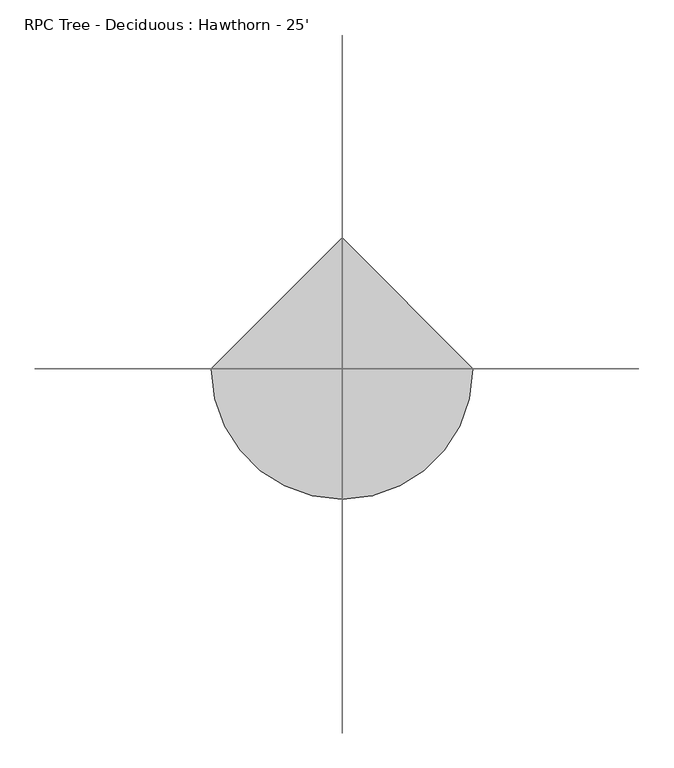
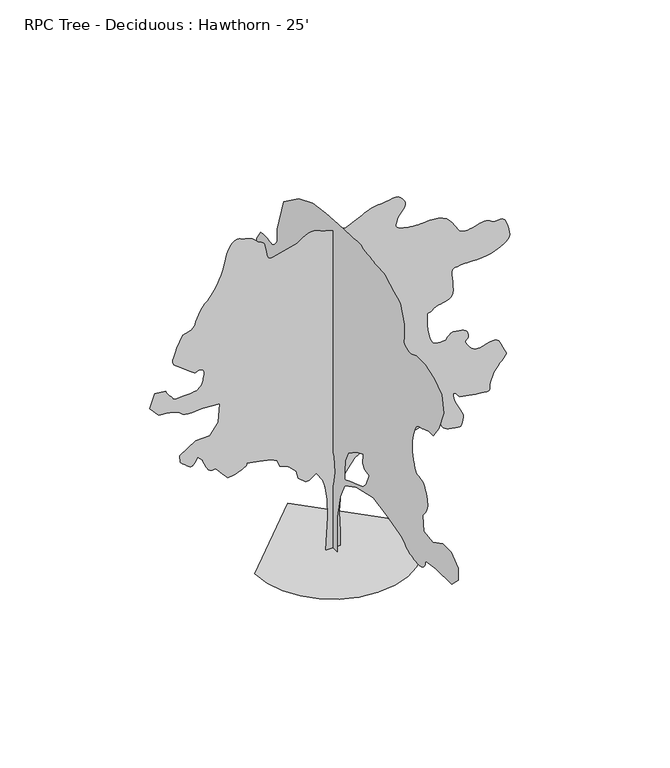
"""IFC4 building model written with IfcOpenShell, lengths in millimetres: geographic element geometry, RPC Tree - Deciduous : Hawthorn - 25'."""

from ifc_helpers import new_model, si_unit, origin, place, context, project, spatial, triangles, source, transform, mapped, element, save


def rpc_tree_deciduous_hawthorn_25_a438f522(model_context):
    return source(origin(), model_context, "Body", "Tessellation", [
        triangles([(159.1331283, 0.0003947, 0.019308), (-154.090976, 0.0003947, 0.019308), (-109.3440979, 0.0003507, 738.3315319), (-120.5310059, 0.000328, 1118.6758307), (-165.2768666, 0.0003107, 1409.5258827), (-210.0237538, 0.0003, 1588.5119053), (-355.4472356, 0.000288, 1789.8701088), (-500.8748051, 0.000294, 1689.1897717), (-579.1803815, 0.0002947, 1678.0035358), (-735.7915707, 0.0002867, 1812.2424351), (-780.538694, 0.000276, 1991.2284576), (-937.1498468, 0.0002667, 2147.8396832), (-1127.3219599, 0.000262, 2226.1452232), (-1183.2552464, 0.000254, 2360.3841225), (-1306.3080551, 0.00025, 2427.5035721), (-1563.5970016, 0.0002467, 2483.4367859), (-1820.8885643, 0.000244, 2528.1814384), (-1818.86674, 0.0002446, 2518.4962738), (-1819.0953598, 0.0002452, 2508.2221916), (-1823.8248676, 0.0002459, 2496.7743439), (-1835.3057076, 0.0002466, 2483.5664291), (-1855.7857075, 0.0002476, 2468.0089485), (-1887.5203983, 0.0002487, 2449.5176353), (-1932.7551373, 0.00025, 2427.5035721), (-1983.2071449, 0.0002513, 2406.1420853), (-2029.5519905, 0.0002523, 2389.4746433), (-2072.4703011, 0.000253, 2376.7238228), (-2112.6530228, 0.0002536, 2367.102317), (-2150.7784573, 0.000254, 2359.8303772), (-2187.5321732, 0.0002544, 2354.1230221), (-2223.605262, 0.0002547, 2349.1978867), (-2346.6579254, 0.0002467, 2483.4367859), (-2480.8968246, 0.0002373, 2640.0478661), (-2507.2492859, 0.0002376, 2635.5522102), (-2533.5026253, 0.0002377, 2632.8090637), (-2559.5553955, 0.0002377, 2633.596225), (-2585.33638, 0.0002373, 2639.6670753), (-2610.710994, 0.0002366, 2652.7732521), (-2635.5774994, 0.0002353, 2674.6934258), (-2659.885318, 0.0002333, 2707.1548164), (-2681.9072296, 0.0002311, 2744.2133102), (-2700.3982521, 0.000229, 2778.9097389), (-2715.9429428, 0.0002271, 2811.6501823), (-2729.1511482, 0.0002252, 2842.8413017), (-2740.6065536, 0.0002234, 2872.8385986), (-2750.8681366, 0.0002217, 2902.0740234), (-2760.570742, 0.00022, 2930.9030777), (-2861.2308769, 0.000214, 3031.5885017), (-2928.3631165, 0.00022, 2930.9030777), (-2940.4789467, 0.0002211, 2912.005394), (-2953.5089653, 0.0002221, 2894.8857994), (-2968.2664948, 0.0002229, 2881.2968033), (-2985.6907219, 0.0002234, 2872.9656258), (-3006.6202583, 0.0002235, 2871.6956451), (-3031.9695831, 0.0002231, 2879.2396614), (-3062.6020157, 0.000222, 2897.3496025), (-3096.5362816, 0.0002205, 2923.0035599), (-3130.1150459, 0.0002188, 2950.6387917), (-3161.5093506, 0.0002172, 2978.0708382), (-3189.0175552, 0.0002157, 3003.1405289), (-3210.8362816, 0.0002144, 3023.7145638), (-3225.212439, 0.0002136, 3037.6337723), (-3230.3940994, 0.0002133, 3042.7645638), (-3241.5701614, 0.000204, 3199.3808762), (-2905.9857033, 0.0001913, 3411.9277863), (-2603.9547203, 0.0001906, 3423.1038483), (-2424.9634655, 0.0001766, 3658.0281715), (-2391.402578, 0.0001526, 4060.7448692), (-2760.570742, 0.0001506, 4094.2980537), (-2839.3868614, 0.0001512, 4085.027108), (-2916.5522095, 0.0001516, 4077.7374367), (-2990.3898537, 0.0001518, 4074.3338654), (-3059.2490227, 0.0001517, 4076.8229576), (-3121.4283669, 0.0001511, 4087.1354095), (-3175.301532, 0.0001499, 4107.2266251), (-3219.2180374, 0.000148, 4139.0528801), (-3263.4394661, 0.0001459, 4173.1650421), (-3318.227401, 0.0001444, 4199.6317406), (-3381.8287514, 0.0001432, 4219.7741158), (-3452.4660095, 0.0001423, 4234.8106979), (-3528.3866661, 0.0001416, 4246.0120491), (-3607.8379211, 0.0001411, 4254.6990189), (-3689.0413948, 0.0001406, 4262.0904282), (-3879.2111824, 0.000128, 4474.6373383), (-3767.3496964, 0.0001106, 4765.4925499), (-3543.6267242, 0.000112, 4743.1151367), (-3529.174118, 0.0001135, 4716.8007545), (-3514.3404305, 0.0001151, 4690.7657158), (-3498.7195816, 0.0001166, 4665.3402328), (-3481.9046196, 0.0001181, 4640.7786507), (-3463.5406242, 0.0001195, 4617.3853111), (-3443.2206436, 0.0001208, 4595.4904266), (-3420.563887, 0.000122, 4575.3227623), (-3403.5713196, 0.0001231, 4556.2983421), (-3395.5956436, 0.0001242, 4538.2642685), (-3389.1692917, 0.0001251, 4522.1861801), (-3376.875856, 0.0001259, 4509.0544235), (-3351.2727676, 0.0001265, 4499.8340561), (-3304.9177483, 0.0001267, 4495.4907166), (-3230.3940994, 0.0001266, 4497.0147514), (-3147.7933273, 0.0001263, 4501.8153305), (-3080.4326134, 0.0001261, 4506.6159096), (-3025.7972855, 0.0001258, 4511.3911995), (-2981.3473824, 0.0001255, 4516.1917786), (-2944.5429428, 0.0001252, 4520.9923576), (-2912.7928459, 0.0001249, 4525.7929367), (-2883.6082901, 0.0001246, 4530.5679359), (-2855.0332901, 0.0001233, 4552.2596352), (-2827.6521126, 0.000122, 4574.6370483), (-2802.607711, 0.0001206, 4598.3858894), (-2781.0686188, 0.0001191, 4624.1668739), (-2764.2539474, 0.0001174, 4652.7165848), (-2753.2810707, 0.0001154, 4684.6695763), (-2749.3693909, 0.0001133, 4720.7377235), (-2745.4071327, 0.0001109, 4760.7934181), (-2736.720163, 0.0001084, 4802.805098), (-2728.2366692, 0.0001059, 4844.6133018), (-2724.858387, 0.0001036, 4884.0850204), (-2731.4370552, 0.0001015, 4919.0352127), (-2752.8999893, 9.98e-05, 4947.3561584), (-2794.1242172, 9.86e-05, 4966.8636887), (-2835.4754723, 9.84e-05, 4971.2320267), (-2860.596032, 9.89e-05, 4962.0883987), (-2879.2396614, 9.97e-05, 4949.2356949), (-2901.2359932, 0.0001001, 4942.4541321), (-2936.3132126, 9.95e-05, 4951.5216019), (-2994.3015335, 9.75e-05, 4986.2183212), (-3084.9794289, 9.33e-05, 5056.3477615), (-3185.5886948, 8.86e-05, 5134.4522964), (-3266.6398521, 8.52e-05, 5192.2121429), (-3327.7268211, 8.25e-05, 5238.0337646), (-3368.4429405, 7.99e-05, 5280.3497864), (-3388.4327087, 7.71e-05, 5327.5178375), (-3387.2897552, 7.35e-05, 5388.0205399), (-3364.6329987, 6.86e-05, 5470.2399399), (-3332.3750839, 6.34e-05, 5558.3020065), (-3302.4792343, 5.9e-05, 5632.2666779), (-3274.5137901, 5.53e-05, 5694.4966003), (-3248.1488297, 5.21e-05, 5747.3282593), (-3222.926532, 4.94e-05, 5793.1248825), (-3198.4916862, 4.69e-05, 5834.2217926), (-3174.4635017, 4.46e-05, 5872.9566376), (-3129.0991196, 4.4e-05, 5882.81185), (-3084.8015327, 4.34e-05, 5894.2163864), (-3042.6628258, 4.25e-05, 5908.7707306), (-3003.7500847, 4.13e-05, 5928.0236252), (-2969.155394, 3.98e-05, 5953.5255569), (-2939.945549, 3.78e-05, 5986.850267), (-2917.1617653, 3.53e-05, 6029.5732407), (-2900.9310699, 3.27e-05, 6072.7020035), (-2888.6120544, 3.06e-05, 6108.7701508), (-2877.258387, 2.86e-05, 6141.7140701), (-2863.9487343, 2.66e-05, 6175.4195709), (-2845.7370552, 2.43e-05, 6213.8497833), (-2819.7273056, 2.15e-05, 6260.8649368), (-2782.9228661, 1.79e-05, 6320.4281616), (-2744.5688118, 1.47e-05, 6374.7841461), (-2713.0727692, 1.26e-05, 6410.1918686), (-2684.3201637, 1.1e-05, 6436.3792236), (-2654.1702599, 9.4e-06, 6463.150264), (-2618.5596428, 7.2e-06, 6500.2852066), (-2573.3475769, 3.8e-06, 6557.5875229), (-2514.4552414, -1.4e-06, 6644.8362671), (-2453.8586494, -7.4e-06, 6746.4620407), (-2405.0042187, -1.31e-05, 6841.4324066), (-2365.9314583, -1.85e-05, 6931.32285), (-2334.6868538, -2.36e-05, 7017.682695), (-2309.3123852, -2.86e-05, 7102.0868454), (-2287.8543926, -3.36e-05, 7186.1102051), (-2268.3497692, -3.87e-05, 7271.2759369), (-2244.5754936, -4.38e-05, 7356.7980423), (-2212.386034, -4.86e-05, 7437.6204346), (-2172.9551559, -5.29e-05, 7509.0451447), (-2127.4586597, -5.63e-05, 7566.3730408), (-2077.0701656, -5.86e-05, 7604.9299896), (-2022.9657646, -5.95e-05, 7619.9924423), (-1966.3136993, -5.87e-05, 7606.8862656), (-1910.121199, -5.73e-05, 7582.9086594), (-1856.4689507, -5.63e-05, 7565.7887741), (-1805.1685936, -5.54e-05, 7551.412326), (-1756.0195587, -5.45e-05, 7535.6644501), (-1708.8265091, -5.32e-05, 7514.4302811), (-1663.3961426, -5.14e-05, 7483.5943726), (-1619.5303608, -4.87e-05, 7439.0936005), (-1579.0555058, -4.63e-05, 7399.0890656), (-1543.670747, -4.51e-05, 7378.0827896), (-1512.9800331, -4.44e-05, 7366.2974625), (-1486.5970505, -4.37e-05, 7353.9022888), (-1464.1256023, -4.23e-05, 7331.1437943), (-1445.1773403, -3.97e-05, 7288.217926), (-1429.3581024, -3.54e-05, 7215.3456299), (-1415.9875523, -3.04e-05, 7132.3890656), (-1403.2038849, -2.64e-05, 7065.2571167), (-1388.8528713, -2.34e-05, 7013.4155136), (-1370.7858055, -2.11e-05, 6976.2299927), (-1346.8464237, -1.98e-05, 6953.1412857), (-1314.8855839, -1.92e-05, 6943.5401276), (-1272.7470222, -1.94e-05, 6946.8678314), (-758.1663677, -2.74e-05, 7081.1067307), (-698.2198814, -2.99e-05, 7123.7785446), (-638.1794329, -3.23e-05, 7163.5040268), (-577.9408496, -3.43e-05, 7197.3368454), (-517.4101693, -3.58e-05, 7222.4068268), (-456.4857994, -3.66e-05, 7235.6908997), (-395.0737412, -3.65e-05, 7234.3444702), (-333.0749456, -3.54e-05, 7215.3456299), (-271.7289263, -3.38e-05, 7188.8786407), (-212.1431193, -3.25e-05, 7166.5015182), (-154.0251915, -3.14e-05, 7147.5526749), (-97.0814925, -3.04e-05, 7131.34785), (-41.0181631, -2.95e-05, 7117.1742966), (14.4578691, -2.88e-05, 7104.3983322), (69.6403804, -2.81e-05, 7092.3077911), (270.9999556, -2.67e-05, 7069.9306686), (584.2222612, -3.47e-05, 7204.1695679), (629.9473045, -3.64e-05, 7232.7445679), (676.749317, -3.81e-05, 7260.1254547), (725.7026516, -3.96e-05, 7285.1698563), (777.8843502, -4.08e-05, 7306.7092392), (834.371382, -4.18e-05, 7323.5239105), (896.2406433, -4.25e-05, 7334.4964966), (964.56656, -4.27e-05, 7338.4084671), (1038.7294024, -4.3e-05, 7343.6912842), (1115.4373655, -4.38e-05, 7356.0102997), (1191.7540735, -4.46e-05, 7370.107695), (1264.743441, -4.52e-05, 7380.6739105), (1331.4717808, -4.54e-05, 7382.4261292), (1389.0027168, -4.46e-05, 7370.107695), (1434.402562, -4.27e-05, 7338.4084671), (1469.8203129, -4.03e-05, 7297.1080811), (1498.5858536, -3.8e-05, 7258.7540268), (1519.5229477, -3.58e-05, 7222.177771), (1531.4610271, -3.37e-05, 7186.1607834), (1533.2212395, -3.15e-05, 7149.5595291), (1523.6327259, -2.92e-05, 7111.2054749), (1501.5195408, -2.67e-05, 7069.9306686), (1474.1255733, -2.45e-05, 7032.3637756), (1449.4698109, -2.28e-05, 7003.585881), (1427.5522533, -2.14e-05, 6980.1163834), (1408.3752262, -2.01e-05, 6958.3991043), (1391.9388748, -1.87e-05, 6934.9040268), (1378.2407284, -1.7e-05, 6906.151712), (1367.2806416, -1.47e-05, 6868.5598206), (1355.7362881, -1.23e-05, 6828.0210159), (1343.4097149, -1.02e-05, 6792.1819244), (1334.9946762, -8.3e-06, 6760.2542221), (1335.1903038, -6.6e-06, 6731.4507477), (1348.692968, -5e-06, 6705.0093384), (1380.1965683, -3.5e-06, 6680.1172531), (1434.402562, -2.1e-06, 6656.0123291), (1502.5633724, -8e-07, 6635.3118484), (1571.509164, 1e-07, 6620.4778702), (1639.2813354, 7e-07, 6610.5209198), (1703.9217213, 1e-06, 6604.5015198), (1763.4744816, 1.2e-06, 6601.4028717), (1815.9839218, 1.3e-06, 6600.2593369), (1859.4914406, 1.3e-06, 6600.0820221), (1908.6404755, 1.1e-06, 6602.7998795), (1975.9885448, 8e-07, 6608.0571167), (2056.4454071, 6e-07, 6611.5371368), (2144.9261982, 8e-07, 6608.9715958), (2236.3432926, 1.5e-06, 6596.0177353), (2325.6064487, 3.2e-06, 6568.3827942), (2407.633128, 5.9e-06, 6521.7734299), (2476.0555504, 9.6e-06, 6460.1789337), (2530.3911873, 1.36e-05, 6393.2754593), (2574.3635033, 1.77e-05, 6325.4063461), (2611.6760513, 2.15e-05, 6260.8649368), (2646.0422676, 2.49e-05, 6203.9689911), (2681.1959358, 2.76e-05, 6158.9856903), (2720.8452599, 2.93e-05, 6130.258374), (2765.3207428, 3.01e-05, 6115.9580841), (2812.1074219, 3.05e-05, 6110.4973709), (2860.8753754, 3.04e-05, 6112.3513275), (2911.1926529, 2.99e-05, 6120.0729492), (2962.6784637, 2.92e-05, 6132.2140686), (3014.9770157, 2.83e-05, 6147.2765213), (3067.6310692, 2.73e-05, 6163.8115585), (3115.4592545, 2.67e-05, 6173.1080841), (3162.4746986, 2.63e-05, 6180.6518097), (3207.9405281, 2.6e-05, 6184.6649368), (3251.0698723, 2.61e-05, 6183.3952469), (3291.0494087, 2.66e-05, 6175.0637787), (3327.1172653, 2.76e-05, 6157.9444748), (3358.4862808, 2.93e-05, 6130.258374), (3393.4620529, 3.05e-05, 6109.9386841), (3438.1912994, 3.06e-05, 6108.7957306), (3488.8135002, 3.01e-05, 6115.881926), (3541.3913956, 2.99e-05, 6120.200267), (3592.0135963, 3.04e-05, 6110.8531631), (3636.7428429, 3.25e-05, 6076.8424484), (3671.718615, 3.66e-05, 6007.1955368), (3699.2776886, 4.18e-05, 5920.2258453), (3722.3408157, 4.65e-05, 5841.4608856), (3737.75877, 5.07e-05, 5770.9250748), (3742.4323219, 5.44e-05, 5708.5934143), (3733.1866653, 5.76e-05, 5654.4914841), (3706.9484413, 6.04e-05, 5608.5937042), (3660.5172638, 6.26e-05, 5570.9256546), (3605.0439056, 6.46e-05, 5537.5247864), (3550.9419754, 6.65e-05, 5505.1145554), (3494.096608, 6.84e-05, 5474.6594376), (3430.3935196, 7e-05, 5447.1262344), (3355.7431343, 7.14e-05, 5423.5044205), (3266.0302963, 7.25e-05, 5404.7846329), (3157.1407219, 7.33e-05, 5391.931929), (3050.6893707, 7.37e-05, 5385.4549988), (2967.1235413, 7.38e-05, 5383.8550964), (2900.6008575, 7.37e-05, 5385.2009445), (2845.2036575, 7.36e-05, 5387.5124313), (2795.1148544, 7.35e-05, 5388.8332809), (2744.4417847, 7.36e-05, 5387.2327972), (2687.2917847, 7.4e-05, 5380.755867), (2632.1995079, 7.44e-05, 5373.8725662), (2590.4418823, 7.46e-05, 5369.5292267), (2560.1905312, 7.5e-05, 5363.4330872), (2539.7510811, 7.57e-05, 5351.2663879), (2527.325386, 7.71e-05, 5328.7369492), (2521.1609367, 7.93e-05, 5291.5258484), (2519.4970848, 8.26e-05, 5235.3409058), (2523.9979729, 8.71e-05, 5159.8269104), (2533.5866318, 9.23e-05, 5072.4002701), (2542.3849319, 9.78e-05, 4980.2494995), (2544.5441025, 0.0001032, 4890.6636887), (2534.1732239, 0.0001079, 4810.8569321), (2505.4078285, 0.0001117, 4748.0680321), (2452.3776352, 0.000114, 4709.5616615), (2387.9658691, 0.0001152, 4689.2416809), (2328.8373562, 0.0001161, 4674.4079933), (2274.7963234, 0.0001168, 4662.2924538), (2225.6474339, 0.0001175, 4650.2019127), (2181.1949146, 0.0001184, 4635.3682251), (2141.2406673, 0.0001196, 4615.0482445), (2105.594442, 0.0001213, 4586.4988243), (2074.7410927, 0.0001226, 4564.2231491), (2049.1734673, 0.000123, 4557.6189011), (2028.6908512, 0.0001231, 4556.2727623), (2013.1029945, 0.0001235, 4549.846701), (2002.2088921, 0.0001248, 4527.9773964), (1995.8156776, 0.0001276, 4480.2506584), (1993.727869, 0.0001326, 4396.3293274), (1998.2947414, 0.000139, 4289.0143661), (2011.0810249, 0.0001454, 4181.4709305), (2030.7126755, 0.0001515, 4079.0327065), (2055.8256775, 0.000157, 3986.9578033), (2085.0483124, 0.0001616, 3910.5546181), (2117.0091522, 0.0001649, 3855.0812599), (2150.3415653, 0.0001666, 3825.8202553), (2188.6294899, 0.0001673, 3814.6444839), (2233.3766132, 0.0001676, 3808.9294258), (2280.0795765, 0.0001677, 3807.3292328), (2324.2399624, 0.0001677, 3808.4721863), (2361.351796, 0.0001675, 3810.9868584), (2386.9220375, 0.0001674, 3813.5015305), (2396.4468922, 0.0001673, 3814.6444839), (2400.0004543, 0.0001668, 3823.2041359), (2411.1865448, 0.0001655, 3844.8958351), (2430.787674, 0.0001638, 3873.6231514), (2459.5862068, 0.000162, 3903.3411049), (2498.3643631, 0.0001605, 3927.9791359), (2547.8968048, 0.0001597, 3941.4411049), (2608.9837738, 0.00016, 3937.6817413), (2671.9758591, 0.0001607, 3924.8296188), (2726.5347382, 0.0001614, 3912.9675522), (2772.483387, 0.0001623, 3898.9468964), (2809.6183296, 0.0001634, 3879.6428421), (2837.7866684, 0.0001651, 3851.906163), (2856.7352211, 0.0001674, 3812.6379204), (2866.2855103, 0.0001706, 3758.7135956), (2862.7040428, 0.0001735, 3709.9456421), (2847.1593521, 0.0001752, 3682.3104103), (2826.9411095, 0.0001761, 3666.8418777), (2809.2625374, 0.0001769, 3654.4722839), (2801.3885994, 0.0001779, 3636.235025), (2810.5072289, 0.0001799, 3603.1387894), (2843.9080971, 0.0001833, 3546.1666855), (2889.3486374, 0.000187, 3484.6480568), (2930.6490234, 0.0001895, 3441.7218979), (2969.2315521, 0.0001912, 3414.061377), (3006.467942, 0.0001921, 3398.3640793), (3043.6790428, 0.0001925, 3391.2523041), (3082.2615715, 0.0001926, 3389.4233459), (3123.5619576, 0.0001926, 3389.5503731), (3174.7428452, 0.0001921, 3399.3294273), (3238.4459335, 0.0001908, 3421.249601), (3309.3628258, 0.0001894, 3444.134832), (3382.2607018, 0.0001886, 3456.860218), (3451.8311646, 0.0001891, 3448.2496971), (3512.7911064, 0.0001916, 3407.1524963), (3559.8571289, 0.0001966, 3322.4181335), (3596.9920715, 0.0002022, 3228.6924591), (3629.6310677, 0.0002061, 3162.9572273), (3654.6498894, 0.0002089, 3117.5419762), (3668.8993103, 0.0002108, 3084.8776909), (3669.2803917, 0.0002124, 3057.2680389), (3652.5924568, 0.0002142, 3027.1437149), (3615.7880173, 0.0002166, 2986.8336754), (3572.5063568, 0.0002193, 2942.3837723), (3537.6831917, 0.0002217, 2904.233194), (3509.8447746, 0.0002237, 2871.3148544), (3487.6196777, 0.0002256, 2842.5872475), (3469.6111839, 0.0002272, 2817.0094482), (3454.4219948, 0.0002288, 2793.5399506), (3440.6298134, 0.0002303, 2771.0863792), (3437.2006622, 0.00023, 2773.5501823), (3432.5271103, 0.0002299, 2772.1278854), (3425.3897552, 0.0002303, 2763.0345451), (3414.5439056, 0.0002314, 2742.4099319), (3398.7451607, 0.0002335, 2706.4182335), (3376.7235397, 0.0002367, 2651.1986389), (3347.3102188, 0.0002413, 2572.9412064), (3325.1359909, 0.0002461, 2493.0582916), (3319.1924583, 0.0002496, 2433.9271626), (3319.7005669, 0.000252, 2392.9976841), (3316.9065514, 0.0002535, 2367.722192), (3300.9807793, 0.0002543, 2355.5581089), (3262.1694855, 0.0002544, 2353.9579159), (3190.6939064, 0.000254, 2360.3841225), (3103.5213203, 0.0002534, 2370.2977615), (3023.3843513, 0.0002528, 2380.8006088), (2949.1147568, 0.0002521, 2391.791217), (2879.544294, 0.0002514, 2403.1729351), (2813.5044296, 0.0002507, 2414.8492573), (2749.8266304, 0.00025, 2426.721207), (2687.2917847, 0.0002493, 2438.6895172), (2647.0584846, 0.0002464, 2487.937674), (2609.8473839, 0.0002438, 2530.6275101), (2578.6815536, 0.0002421, 2560.2158203), (2556.6343529, 0.0002415, 2570.1219017), (2546.7285622, 0.0002425, 2553.8150482), (2551.9863808, 0.0002454, 2504.7319977), (2575.4302986, 0.0002507, 2416.3173363), (2612.9463226, 0.0002568, 2313.8436493), (2654.9324226, 0.000262, 2225.2638817), (2696.3598358, 0.0002666, 2148.0351654), (2732.09748, 0.0002707, 2079.6102722), (2757.0910126, 0.0002744, 2017.4488049), (2766.209642, 0.0002779, 1959.0060059), (2754.4240242, 0.0002813, 1901.734211), (2736.8980591, 0.0002844, 1850.8910934), (2728.0081947, 0.0002866, 1812.7631882), (2721.2516304, 0.0002882, 1786.3802055), (2710.2025955, 0.0002891, 1770.7567406), (2688.3841599, 0.0002895, 1764.9197422), (2649.3443916, 0.0002893, 1767.8864216), (2586.6063606, 0.0002887, 1778.6815475), (2516.4972679, 0.0002878, 1792.6413059), (2458.5092377, 0.000287, 1806.7966919), (2411.0875683, 0.000286, 1822.7122902), (2372.6700005, 0.0002849, 1841.9528309), (2341.6871532, 0.0002834, 1866.0878403), (2316.5741512, 0.0002816, 1896.6795776), (2295.766555, 0.0002793, 1935.2952438), (2282.6220085, 0.0002768, 1976.9435738), (2278.2862267, 0.0002746, 2015.0688629), (2277.8621246, 0.0002726, 2048.8888916), (2276.46003, 0.0002708, 2077.6214401), (2269.185474, 0.0002695, 2100.4838528), (2251.1515457, 0.0002685, 2116.6915844), (2217.4610149, 0.000268, 2125.4673569), (2177.5728973, 0.0002678, 2129.2823856), (2143.5572411, 0.0002676, 2131.3372021), (2114.4335827, 0.0002676, 2131.9239395), (2089.2216042, 0.0002676, 2131.3372021), (2066.9483997, 0.0002677, 2129.8691231), (2046.6284191, 0.0002678, 2127.8143066), (2027.2887566, 0.000268, 2125.4673569), (1758.8111034, 0.000274, 2024.7868744), (1579.8250809, 0.0002667, 2147.8396832), (1380.9128036, 0.0002704, 2075.457328), (1410.85429, 0.0002716, 2057.3014595), (1436.60984, 0.0002729, 2038.5130714), (1453.9936626, 0.0002741, 2018.4597897), (1458.8195309, 0.0002755, 1996.5066238), (1446.9019444, 0.0002771, 1972.0210545), (1414.0572922, 0.0002788, 1944.370562), (1356.0970219, 0.0002807, 1912.9203014), (1293.4784603, 0.0002823, 1885.3308517), (1245.5334217, 0.0002833, 1868.8920296), (1206.3972204, 0.0002837, 1862.4353016), (1170.1971771, 0.0002835, 1864.7822514), (1131.0609032, 0.0002829, 1874.7644909), (1083.118408, 0.0002819, 1891.2008423), (1020.4998465, 0.0002807, 1912.9203014), (729.6473236, 0.0002753, 2002.4145481), (461.1695615, 0.000284, 1856.9895584), (259.8112671, 0.0003, 1588.5119053), (192.6930892, 0.0003113, 1398.3397923), (170.3192732, 0.0003253, 1163.422954), (136.7603205, 0.0003487, 771.8924921), (159.1331283, 0.0003767, 302.0564901), (-0.000123, -157.488225, 0.0160584), (-0.000123, 166.924822, 0.0160778), (-0.0001013, 177.738606, 702.9113102), (-8.68e-05, 231.8072715, 1059.765691), (-7.23e-05, 404.8273247, 1416.6200718), (-6.51e-05, 567.0341025, 1654.5213936), (-5.79e-05, 848.1915413, 1849.1689602), (-4.34e-05, 1334.8118385, 2065.4447124), (-2.89e-05, 1907.9419716, 2130.3263626), (-2.89e-05, 2243.1683121, 1924.8659386), (-2.89e-05, 2491.8848167, 1892.4250408), (-2.17e-05, 2632.4532715, 2162.7697311), (-1.45e-05, 2859.5545258, 2195.2106289), (-7.2e-06, 3335.3469955, 2227.6513813), (0.0, 3616.5246002, 2249.279567), (7.2e-06, 3757.0881134, 2357.4172977), (7.2e-06, 3746.2931328, 2530.436824), (1.45e-05, 3919.2921661, 2638.5747002), (1.45e-05, 3967.7046181, 2647.972673), (1.45e-05, 4014.4912971, 2658.1328087), (1.45e-05, 4058.052301, 2669.7913994), (2.17e-05, 4096.7874367, 2683.7106079), (2.17e-05, 4129.1215096, 2700.6775955), (2.17e-05, 4153.3784592, 2721.4295265), (2.17e-05, 4168.0089615, 2746.7024025), (2.17e-05, 4176.6447716, 2777.0299118), (2.17e-05, 4184.163208, 2811.9042366), (2.17e-05, 4190.7162964, 2850.5629234), (2.89e-05, 4196.5075127, 2892.2443909), (2.89e-05, 4201.7400421, 2936.1861855), (2.89e-05, 4206.6167793, 2981.6523056), (2.89e-05, 4211.2650421, 3027.8802979), (3.62e-05, 4027.4454483, 3254.9559723), (2.89e-05, 3627.3195808, 3276.5968025), (2.17e-05, 3389.4233459, 3103.5721893), (2.17e-05, 3374.8945816, 3100.7020157), (2.17e-05, 3336.7184235, 3093.8440041), (2.17e-05, 3283.0228638, 3085.690432), (1.45e-05, 3221.9614746, 3078.8580002), (1.45e-05, 3161.6363777, 3075.9878265), (1.45e-05, 3110.2270157, 3079.7216103), (1.45e-05, 3075.8352196, 3092.7516289), (1.45e-05, 3052.3404327, 3114.7479607), (1.45e-05, 3028.2866684, 3143.0183281), (1.45e-05, 3003.7500847, 3176.4444855), (1.45e-05, 2978.8582901, 3214.0619568), (2.17e-05, 2953.6615723, 3254.803656), (2.17e-05, 2928.2869583, 3297.6277863), (2.17e-05, 2902.8106064, 3341.4681335), (2.89e-05, 2848.734256, 3611.8254684), (3.62e-05, 3075.8352196, 3784.8247925), (5.06e-05, 3248.8598328, 4076.7976685), (5.06e-05, 2967.6822281, 4336.3344429), (4.34e-05, 2675.7096428, 4239.0017212), (3.62e-05, 2491.8848167, 4087.6179382), (3.62e-05, 2286.4219219, 4228.2067406), (4.34e-05, 2286.4219219, 4466.1029755), (5.79e-05, 2481.0694885, 4682.3836693), (5.79e-05, 2522.6544502, 4705.5229546), (5.79e-05, 2563.4923645, 4728.4593452), (5.79e-05, 2602.786187, 4751.0399437), (5.79e-05, 2639.8446808, 4773.0362755), (5.79e-05, 2673.8553955, 4794.2960243), (6.51e-05, 2704.0811668, 4814.5907158), (6.51e-05, 2729.7859932, 4833.7674522), (6.51e-05, 2749.8013412, 4860.5137848), (6.51e-05, 2764.1522095, 4901.992067), (6.51e-05, 2773.7789474, 4955.7887833), (7.23e-05, 2779.5954529, 5019.390715), (7.23e-05, 2782.5926537, 5090.4090546), (7.23e-05, 2783.710318, 5166.3038406), (7.23e-05, 2783.8626343, 5244.688591), (7.96e-05, 2643.2738319, 5460.9689941), (7.96e-05, 2638.1936188, 5462.1375275), (7.96e-05, 2623.8680397, 5465.0077011), (7.96e-05, 2601.5670753, 5468.6400375), (7.96e-05, 2572.6618629, 5472.068898), (7.96e-05, 2538.4505791, 5474.354805), (7.96e-05, 2500.2694794, 5474.5832794), (7.96e-05, 2459.4440643, 5471.7892639), (7.96e-05, 2416.0634274, 5465.5158096), (7.23e-05, 2370.5999233, 5457.3366577), (7.23e-05, 2324.9486401, 5449.3615631), (7.23e-05, 2281.0014679, 5443.6462143), (7.23e-05, 2240.6460823, 5442.3003662), (7.23e-05, 2205.7769897, 5447.3802887), (7.23e-05, 2178.2865166, 5460.9689941), (7.23e-05, 2156.0590942, 5480.4509445), (7.23e-05, 2135.5359283, 5501.6345352), (7.23e-05, 2116.4299725, 5524.2407135), (7.23e-05, 2098.4595577, 5547.9892639), (7.23e-05, 2081.3399632, 5572.5767166), (7.23e-05, 2064.7867584, 5597.7228561), (7.23e-05, 2048.5206001, 5623.1736282), (8.68e-05, 2037.7052719, 5893.5053833), (0.0001013, 1810.6168076, 6650.4754578), (0.0001085, 1259.1148602, 7050.6010345), (0.0001085, 740.0536652, 7266.8564392), (0.0001013, 264.2486416, 7331.7536407), (9.4e-05, -200.7431066, 7364.1894516), (8.68e-05, -654.9205622, 7385.8299911), (8.68e-05, -694.7400793, 7388.0908997), (8.68e-05, -753.6629362, 7393.3737167), (8.68e-05, -824.3155277, 7399.4442764), (8.68e-05, -899.3190891, 7403.9655121), (8.68e-05, -971.295001, 7404.7276749), (7.96e-05, -1032.8671148, 7399.4442764), (7.96e-05, -1076.6592093, 7385.8299911), (7.96e-05, -1121.7111105, 7368.5327911), (7.96e-05, -1186.8138227, 7353.5464966), (7.96e-05, -1264.2126595, 7340.41474), (7.96e-05, -1346.1503906, 7328.807309), (7.23e-05, -1424.8724751, 7318.3422501), (7.23e-05, -1492.6244442, 7308.6393539), (7.23e-05, -1541.6489227, 7299.3178299), (7.23e-05, -1586.6069344, 7292.8658981), (7.23e-05, -1644.4273876, 7290.2247803), (7.23e-05, -1710.7593853, 7288.5225586), (6.51e-05, -1781.254501, 7284.9413818), (6.51e-05, -1851.5590759, 7276.6099136), (6.51e-05, -1917.3246838, 7260.7097214), (6.51e-05, -1974.2002819, 7234.4206284), (6.51e-05, -2029.2775887, 7201.04534), (5.79e-05, -2091.7336601, 7165.9422501), (5.79e-05, -2160.3364494, 7129.4427338), (5.79e-05, -2233.8566711, 7091.7996826), (5.06e-05, -2311.0675106, 7053.2933121), (5.06e-05, -2390.7344501, 7014.2282547), (5.06e-05, -2471.6334366, 6974.8835632), (3.62e-05, -2623.0300095, 6596.4241058), (2.17e-05, -2612.209449, 6250.3748795), (2.17e-05, -2603.3448738, 6234.0683167), (2.17e-05, -2596.9441017, 6217.3042236), (2.17e-05, -2595.4709358, 6199.5750732), (2.17e-05, -2601.3638901, 6180.4489151), (2.17e-05, -2617.1117661, 6159.4176407), (2.17e-05, -2645.1280792, 6136.0243011), (2.17e-05, -2687.9016312, 6109.7863678), (2.17e-05, -2739.2095459, 6088.9329895), (1.45e-05, -2791.0761475, 6080.5253632), (1.45e-05, -2843.4002792, 6082.5572159), (1.45e-05, -2896.1052017, 6092.894957), (1.45e-05, -2949.1147568, 6109.4811539), (1.45e-05, -3002.3024986, 6130.2327942), (1.45e-05, -3055.5661079, 6153.0424484), (7.2e-06, -3390.7950645, 6153.0424484), (0.0, -3726.0237305, 6044.9147461), (-7.2e-06, -3996.3810654, 5850.2743011), (-2.17e-05, -4061.2526871, 5471.7892639), (-2.89e-05, -3877.4330933, 5017.6123352), (-3.62e-05, -3682.7676498, 4747.255291), (-3.62e-05, -3647.7410088, 4747.0773949), (-3.62e-05, -3611.1144653, 4745.7565453), (-3.62e-05, -3571.261956, 4742.1497887), (-3.62e-05, -3526.5832878, 4735.1647499), (-3.62e-05, -3475.4785583, 4723.6078972), (-3.62e-05, -3416.3472839, 4706.4121445), (-2.89e-05, -3347.5389839, 4682.3836693), (-2.89e-05, -3278.5272079, 4659.244384), (-2.89e-05, -3219.1674591, 4642.9122414), (-2.89e-05, -3168.4943893, 4629.6025887), (-2.89e-05, -3125.5938103, 4615.5310638), (-2.89e-05, -3089.5003738, 4596.9383034), (-2.89e-05, -3059.2746025, 4570.0143654), (-2.89e-05, -3033.9508575, 4530.9745972), (-3.62e-05, -3009.1605103, 4474.9675507), (-3.62e-05, -2982.6935211, 4403.2379173), (-3.62e-05, -2956.7602203, 4321.29757), (-3.62e-05, -2933.6970932, 4234.6330925), (-4.34e-05, -2915.7138885, 4148.7301964), (-4.34e-05, -2905.1220932, 4069.0504669), (-4.34e-05, -2904.182325, 4001.1054863), (-5.06e-05, -2913.1739273, 3931.6111816), (-5.06e-05, -2929.7092552, 3849.0868584), (-5.06e-05, -2952.1375374, 3761.6346382), (-5.79e-05, -2978.7056831, 3677.3828041), (-5.79e-05, -3007.7379227, 3604.510508), (-6.51e-05, -3037.5320343, 3551.0942917), (-6.51e-05, -3066.3866684, 3525.3133072), (-6.51e-05, -3100.752594, 3518.1250832), (-6.51e-05, -3145.3295242, 3512.8163956), (-6.51e-05, -3195.7741196, 3506.0092529), (-6.51e-05, -3247.7424591, 3494.2745041), (-6.51e-05, -3296.840625, 3474.2338669), (-7.23e-05, -3338.775856, 3442.4584808), (-7.23e-05, -3369.1795235, 3395.5447746), (-7.23e-05, -3392.7507591, 3341.163501), (-7.23e-05, -3416.1440987, 3288.8393692), (-7.96e-05, -3437.8357979, 3238.0648521), (-7.96e-05, -3456.3268204, 3188.2048141), (-7.96e-05, -3470.0684235, 3138.7511467), (-7.96e-05, -3477.5612801, 3089.0940033), (-8.68e-05, -3477.3072258, 3038.6752785), (-8.68e-05, -3468.5696777, 2989.2721893), (-8.68e-05, -3452.4660095, 2942.7139847), (-8.68e-05, -3430.2159142, 2898.5181358), (-8.68e-05, -3403.0379219, 2856.2018234), (-8.68e-05, -3372.1767242, 2815.3078079), (-8.68e-05, -3338.8520142, 2775.3791405), (-8.68e-05, -3304.2826126, 2735.9074219), (-0.0001013, -3325.9234428, 2389.8581955), (-0.0001085, -3671.9726692, 2346.6021149), (-0.0001085, -4028.8168762, 2530.436824), (-0.0001085, -4342.4050026, 2530.436824), (-0.000123, -4591.1215073, 2324.9765453), (-0.0001302, -4601.9420677, 2065.4447124), (-0.0001302, -4353.225563, 1827.5433907), (-0.000123, -3769.2801018, 1816.7280624), (-0.000123, -3401.6153343, 1762.6591244), (-0.000123, -3391.887149, 1716.5988544), (-0.000123, -3379.2887901, 1672.2403702), (-0.000123, -3361.0515312, 1631.287928), (-0.000123, -3334.2802002, 1595.4409882), (-0.000123, -3296.1546204, 1566.4036617), (-0.000123, -3243.8560684, 1545.8804958), (-0.000123, -3174.5396599, 1535.57066), (-0.000123, -3100.1939072, 1534.0567989), (-0.000123, -3033.9761467, 1538.0293762), (-0.000123, -2974.7687141, 1546.3529961), (-0.0001157, -2921.4289467, 1557.8922626), (-0.0001157, -2872.8133095, 1571.5116348), (-0.0001157, -2827.8044289, 1586.0760075), (-0.0001157, -2785.2343529, 1600.4524555), (-0.0001157, -2741.7495071, 1620.3151966), (-0.0001157, -2695.6229622, 1649.4464127), (-0.0001085, -2648.1758583, 1683.8735264), (-0.0001085, -2600.7287544, 1719.6265766), (-0.0001085, -2554.6025002, 1752.7277538), (-0.0001085, -2511.138002, 1779.2123291), (-0.0001085, -2471.6334366, 1795.1000221), (-9.4e-05, -1963.3875698, 1935.6812668), (-8.68e-05, -1487.5799847, 2022.1911026), (-7.96e-05, -849.5682014, 1870.7970005), (-7.96e-05, -427.8320978, 1643.7085361), (-8.68e-05, -265.62532, 1308.4821957), (-0.0001013, -157.488225, 789.4210733), (-0.0001157, -157.488225, 356.8696415), (7.2e-06, 350.7584229, 2173.5824432), (7.2e-06, 383.199248, 1989.7475887), (0.0, 350.7584229, 1751.8464123), (-1.45e-05, 220.9934875, 1513.9426197), (-2.17e-05, 69.6010114, 1178.7162792), (-2.17e-05, -27.7230557, 1438.2456413), (-7.2e-06, -81.7917281, 1741.0310841), (0.0, -49.3503716, 2065.4447124), (7.2e-06, 69.6010114, 2314.1612171), (1.45e-05, 177.738606, 2400.6709076), (-3.62e-05, -1109.1000343, 2768.3432327), (-3.62e-05, -860.3835297, 2660.1902412), (-3.62e-05, -568.410799, 2465.5553192), (-4.34e-05, -460.2729229, 2227.6513813), (-5.06e-05, -438.6448462, 1978.9348766), (-5.79e-05, -438.6448462, 1795.1000221), (-5.79e-05, -611.6669523, 1859.9842884), (-5.79e-05, -903.6371395, 1957.3068363), (-5.79e-05, -1109.1000343, 2043.8191429), (-5.79e-05, -1217.2379105, 2162.7697311), (-5.06e-05, -1325.3757866, 2411.4862358), (-4.34e-05, -1163.1689724, 2454.739991), (-4.34e-05, -1098.2847061, 2562.8828087), (-1650.2489799, 0.0, 9.84e-05), (-1606.6219917, -378.1268832, 7.58e-05), (-1482.373035, -725.3775261, 5.51e-05), (-1287.4484505, -1031.8003195, 3.69e-05), (-1031.8003195, -1287.4484505, 2.16e-05), (-725.3775261, -1482.3704189, 1e-05), (-378.1268832, -1606.6219917, 2.6e-06), (6.51e-05, -1650.2489799, 0.0), (378.1268832, -1606.6219917, 2.6e-06), (725.3775261, -1482.3704189, 1e-05), (1031.8003195, -1287.4484505, 2.16e-05), (1287.4484505, -1031.8003195, 3.69e-05), (1482.3704189, -725.3775261, 5.51e-05), (1606.6219917, -378.1268832, 7.58e-05), (1650.2489799, 0.0001443, 9.84e-05), (-0.0002242, 1650.2489799, 0.0001967)], [[403, 404, 405], [1, 2, 3], [491, 1, 3], [490, 491, 3], [490, 3, 4], [489, 490, 4], [489, 4, 5], [488, 489, 5], [84, 85, 86], [84, 86, 87], [83, 84, 87], [83, 87, 88], [83, 88, 89], [83, 89, 90], [82, 83, 90], [82, 90, 91], [82, 91, 92], [81, 82, 92], [81, 92, 93], [81, 93, 94], [81, 94, 95], [81, 95, 96], [81, 96, 97], [80, 81, 97], [80, 97, 98], [79, 80, 98], [79, 98, 99], [78, 79, 99], [78, 99, 100], [77, 78, 100], [77, 100, 101], [488, 5, 6], [487, 488, 6], [76, 77, 101], [76, 101, 102], [75, 76, 102], [74, 75, 102], [73, 74, 102], [73, 102, 103], [72, 73, 103], [72, 103, 104], [71, 72, 104], [71, 104, 105], [70, 71, 105], [70, 105, 106], [70, 106, 107], [69, 70, 107], [68, 69, 107], [68, 107, 108], [68, 108, 109], [68, 109, 110], [68, 110, 111], [68, 111, 112], [63, 64, 65], [62, 63, 65], [61, 62, 65], [60, 61, 65], [59, 60, 65], [58, 59, 65], [57, 58, 65], [56, 57, 65], [55, 56, 65], [54, 55, 65], [53, 54, 65], [52, 53, 65], [51, 52, 65], [50, 51, 65], [49, 50, 65], [48, 49, 65], [48, 65, 66], [47, 48, 66], [30, 31, 32], [467, 468, 469], [487, 6, 7], [486, 487, 7], [68, 112, 113], [8, 9, 10], [7, 8, 10], [7, 10, 11], [29, 30, 32], [414, 415, 416], [414, 416, 417], [413, 414, 417], [413, 417, 418], [412, 413, 418], [412, 418, 419], [141, 142, 143], [411, 412, 419], [411, 419, 420], [12, 13, 14], [28, 29, 32], [424, 425, 426], [27, 28, 32], [442, 443, 444], [441, 442, 444], [441, 444, 445], [440, 441, 445], [440, 445, 446], [439, 440, 446], [439, 446, 447], [438, 439, 447], [437, 438, 447], [436, 437, 447], [436, 447, 448], [435, 436, 448], [435, 448, 449], [435, 449, 450], [435, 450, 451], [435, 451, 452], [435, 452, 453], [435, 453, 454], [435, 454, 455], [435, 455, 456], [434, 435, 456], [434, 456, 457], [433, 434, 457], [433, 457, 458], [432, 433, 458], [432, 458, 459], [431, 432, 459], [431, 459, 460], [431, 460, 461], [430, 431, 461], [430, 461, 462], [430, 462, 463], [430, 463, 464], [411, 420, 421], [410, 411, 421], [410, 421, 422], [409, 410, 422], [409, 422, 423], [408, 409, 423], [408, 423, 424], [408, 424, 426], [408, 426, 427], [408, 427, 428], [407, 408, 428], [430, 464, 465], [406, 407, 428], [473, 474, 475], [472, 473, 475], [472, 475, 476], [471, 472, 476], [471, 476, 477], [470, 471, 477], [470, 477, 478], [470, 478, 479], [470, 479, 480], [470, 480, 481], [470, 481, 482], [470, 482, 483], [470, 483, 484], [470, 484, 485], [406, 428, 429], [26, 27, 32], [68, 113, 114], [25, 26, 32], [25, 32, 33], [24, 25, 33], [23, 24, 33], [22, 23, 33], [21, 22, 33], [20, 21, 33], [19, 20, 33], [18, 19, 33], [17, 18, 33], [46, 47, 66], [430, 465, 466], [45, 46, 66], [44, 45, 66], [43, 44, 66], [42, 43, 66], [41, 42, 66], [40, 41, 66], [39, 40, 66], [38, 39, 66], [37, 38, 66], [36, 37, 66], [35, 36, 66], [34, 35, 66], [33, 34, 66], [17, 33, 66], [17, 66, 67], [16, 17, 67], [15, 16, 67], [15, 67, 68], [68, 114, 115], [68, 115, 116], [68, 116, 117], [430, 466, 467], [430, 467, 469], [429, 430, 469], [403, 405, 406], [124, 125, 126], [123, 124, 126], [123, 126, 127], [403, 406, 429], [402, 403, 429], [401, 402, 429], [400, 401, 429], [399, 400, 429], [122, 123, 127], [122, 127, 128], [486, 7, 11], [486, 11, 12], [485, 486, 12], [485, 12, 14], [394, 395, 396], [393, 394, 396], [393, 396, 397], [392, 393, 397], [392, 397, 398], [391, 392, 398], [391, 398, 399], [391, 399, 429], [390, 391, 429], [389, 390, 429], [388, 389, 429], [387, 388, 429], [386, 387, 429], [385, 386, 429], [384, 385, 429], [383, 384, 429], [382, 383, 429], [381, 382, 429], [380, 381, 429], [379, 380, 429], [378, 379, 429], [377, 378, 429], [376, 377, 429], [376, 429, 469], [375, 376, 469], [374, 375, 469], [374, 469, 470], [374, 470, 485], [374, 485, 14], [373, 374, 14], [373, 14, 15], [373, 15, 68], [373, 68, 117], [373, 117, 118], [373, 118, 119], [372, 373, 119], [372, 119, 120], [325, 326, 327], [325, 327, 328], [324, 325, 328], [323, 324, 328], [323, 328, 329], [323, 329, 330], [322, 323, 330], [322, 330, 331], [321, 322, 331], [321, 331, 332], [320, 321, 332], [320, 332, 333], [319, 320, 333], [175, 176, 177], [174, 175, 177], [173, 174, 177], [173, 177, 178], [172, 173, 178], [172, 178, 179], [171, 172, 179], [170, 171, 179], [170, 179, 180], [170, 180, 181], [170, 181, 182], [170, 182, 183], [170, 183, 184], [169, 170, 184], [169, 184, 185], [168, 169, 185], [168, 185, 186], [167, 168, 186], [166, 167, 186], [166, 186, 187], [166, 187, 188], [166, 188, 189], [166, 189, 190], [166, 190, 191], [166, 191, 192], [166, 192, 193], [166, 193, 194], [166, 194, 195], [165, 166, 195], [164, 165, 195], [164, 195, 196], [163, 164, 196], [162, 163, 196], [162, 196, 197], [161, 162, 197], [160, 161, 197], [289, 290, 291], [289, 291, 292], [288, 289, 292], [288, 292, 293], [287, 288, 293], [287, 293, 294], [286, 287, 294], [286, 294, 295], [286, 295, 296], [286, 296, 297], [286, 297, 298], [286, 298, 299], [286, 299, 300], [286, 300, 301], [286, 301, 302], [286, 302, 303], [286, 303, 304], [286, 304, 305], [286, 305, 306], [285, 286, 306], [285, 306, 307], [284, 285, 307], [283, 284, 307], [282, 283, 307], [281, 282, 307], [280, 281, 307], [279, 280, 307], [278, 279, 307], [277, 278, 307], [276, 277, 307], [275, 276, 307], [275, 307, 308], [275, 308, 309], [274, 275, 309], [274, 309, 310], [273, 274, 310], [273, 310, 311], [273, 311, 312], [272, 273, 312], [272, 312, 313], [271, 272, 313], [271, 313, 314], [271, 314, 315], [271, 315, 316], [270, 271, 316], [270, 316, 317], [269, 270, 317], [268, 269, 317], [267, 268, 317], [266, 267, 317], [265, 266, 317], [264, 265, 317], [263, 264, 317], [262, 263, 317], [261, 262, 317], [260, 261, 317], [259, 260, 317], [258, 259, 317], [257, 258, 317], [256, 257, 317], [256, 317, 318], [255, 256, 318], [254, 255, 318], [253, 254, 318], [252, 253, 318], [252, 318, 319], [252, 319, 333], [252, 333, 334], [252, 334, 335], [252, 335, 336], [252, 336, 337], [252, 337, 338], [251, 252, 338], [250, 251, 338], [249, 250, 338], [249, 338, 339], [248, 249, 339], [369, 370, 371], [369, 371, 372], [368, 369, 372], [367, 368, 372], [366, 367, 372], [365, 366, 372], [364, 365, 372], [363, 364, 372], [362, 363, 372], [361, 362, 372], [360, 361, 372], [359, 360, 372], [358, 359, 372], [357, 358, 372], [356, 357, 372], [355, 356, 372], [354, 355, 372], [248, 339, 340], [140, 141, 143], [140, 143, 144], [139, 140, 144], [353, 354, 372], [132, 133, 134], [131, 132, 134], [131, 134, 135], [130, 131, 135], [130, 135, 136], [129, 130, 136], [129, 136, 137], [128, 129, 137], [122, 128, 137], [122, 137, 138], [122, 138, 139], [122, 139, 144], [122, 144, 145], [122, 145, 146], [121, 122, 146], [121, 146, 147], [120, 121, 147], [120, 147, 148], [120, 148, 149], [120, 149, 150], [120, 150, 151], [120, 151, 152], [120, 152, 153], [120, 153, 154], [120, 154, 155], [120, 155, 156], [120, 156, 157], [120, 157, 158], [120, 158, 159], [120, 159, 160], [120, 160, 197], [120, 197, 198], [120, 198, 199], [227, 228, 229], [227, 229, 230], [226, 227, 230], [226, 230, 231], [225, 226, 231], [225, 231, 232], [225, 232, 233], [225, 233, 234], [225, 234, 235], [225, 235, 236], [225, 236, 237], [225, 237, 238], [225, 238, 239], [225, 239, 240], [224, 225, 240], [224, 240, 241], [223, 224, 241], [223, 241, 242], [222, 223, 242], [222, 242, 243], [222, 243, 244], [222, 244, 245], [221, 222, 245], [220, 221, 245], [219, 220, 245], [218, 219, 245], [218, 245, 246], [217, 218, 246], [216, 217, 246], [215, 216, 246], [215, 246, 247], [214, 215, 247], [214, 247, 248], [214, 248, 340], [213, 214, 340], [212, 213, 340], [211, 212, 340], [211, 340, 341], [210, 211, 341], [209, 210, 341], [209, 341, 342], [208, 209, 342], [207, 208, 342], [207, 342, 343], [206, 207, 343], [205, 206, 343], [204, 205, 343], [203, 204, 343], [202, 203, 343], [201, 202, 343], [200, 201, 343], [199, 200, 343], [120, 199, 343], [120, 343, 344], [120, 344, 345], [120, 345, 346], [120, 346, 347], [120, 347, 348], [352, 353, 372], [351, 352, 372], [350, 351, 372], [349, 350, 372], [349, 372, 120], [349, 120, 348], [733, 741, 742], [741, 733, 734], [492, 731, 732], [492, 732, 733], [728, 492, 733], [727, 728, 733], [741, 734, 735], [733, 742, 743], [733, 743, 744], [741, 735, 736], [726, 727, 733], [726, 733, 744], [725, 726, 744], [724, 725, 744], [724, 744, 745], [724, 745, 746], [723, 724, 746], [723, 746, 747], [723, 747, 748], [741, 736, 737], [492, 493, 494], [723, 748, 749], [542, 543, 544], [542, 544, 545], [541, 542, 545], [541, 545, 546], [501, 502, 503], [500, 501, 503], [722, 723, 749], [506, 507, 508], [505, 506, 508], [641, 642, 643], [741, 737, 738], [696, 697, 698], [695, 696, 698], [695, 698, 699], [694, 695, 699], [693, 694, 699], [693, 699, 700], [692, 693, 700], [523, 524, 525], [522, 523, 525], [521, 522, 525], [521, 525, 526], [520, 521, 526], [519, 520, 526], [518, 519, 526], [517, 518, 526], [516, 517, 526], [515, 516, 526], [514, 515, 526], [513, 514, 526], [512, 513, 526], [511, 512, 526], [510, 511, 526], [509, 510, 526], [508, 509, 526], [505, 508, 526], [505, 526, 527], [505, 527, 528], [505, 528, 529], [505, 529, 530], [504, 505, 530], [504, 530, 531], [504, 531, 532], [504, 532, 533], [503, 504, 533], [503, 533, 534], [503, 534, 535], [500, 503, 535], [500, 535, 536], [500, 536, 537], [500, 537, 538], [500, 538, 539], [500, 539, 540], [500, 540, 541], [500, 541, 546], [500, 546, 547], [499, 500, 547], [641, 643, 644], [638, 639, 640], [638, 640, 641], [637, 638, 641], [637, 641, 644], [637, 644, 645], [637, 645, 646], [636, 637, 646], [636, 646, 647], [635, 636, 647], [634, 635, 647], [634, 647, 648], [634, 648, 649], [633, 634, 649], [633, 649, 650], [633, 650, 651], [632, 633, 651], [632, 651, 652], [632, 652, 653], [631, 632, 653], [631, 653, 654], [630, 631, 654], [630, 654, 655], [629, 630, 655], [629, 655, 656], [628, 629, 656], [749, 750, 751], [749, 751, 739], [563, 564, 565], [563, 565, 566], [563, 566, 567], [563, 567, 568], [563, 568, 569], [562, 563, 569], [562, 569, 570], [562, 570, 571], [562, 571, 572], [561, 562, 572], [561, 572, 573], [561, 573, 574], [560, 561, 574], [559, 560, 574], [559, 574, 575], [558, 559, 575], [557, 558, 575], [556, 557, 575], [555, 556, 575], [554, 555, 575], [553, 554, 575], [552, 553, 575], [551, 552, 575], [550, 551, 575], [549, 550, 575], [549, 575, 576], [549, 576, 577], [548, 549, 577], [548, 577, 578], [548, 578, 579], [498, 499, 547], [619, 620, 621], [628, 656, 657], [627, 628, 657], [586, 587, 588], [548, 579, 580], [618, 619, 621], [618, 621, 622], [618, 622, 623], [617, 618, 623], [617, 623, 624], [616, 617, 624], [615, 616, 624], [586, 588, 589], [585, 586, 589], [585, 589, 590], [585, 590, 591], [585, 591, 592], [627, 657, 658], [615, 624, 625], [614, 615, 625], [548, 580, 581], [498, 547, 548], [498, 548, 581], [498, 581, 582], [498, 582, 583], [498, 583, 584], [498, 584, 585], [498, 585, 592], [498, 592, 593], [497, 498, 593], [497, 593, 594], [497, 594, 595], [497, 595, 596], [497, 596, 597], [497, 597, 598], [497, 598, 599], [497, 599, 600], [497, 600, 601], [497, 601, 602], [497, 602, 603], [497, 603, 604], [497, 604, 605], [497, 605, 606], [497, 606, 607], [497, 607, 608], [497, 608, 609], [627, 658, 659], [613, 614, 625], [612, 613, 625], [611, 612, 625], [610, 611, 625], [609, 610, 625], [740, 741, 738], [626, 627, 659], [626, 659, 660], [722, 749, 739], [721, 722, 739], [609, 625, 626], [609, 626, 660], [609, 660, 661], [609, 661, 662], [609, 662, 663], [675, 676, 677], [674, 675, 677], [674, 677, 678], [673, 674, 678], [672, 673, 678], [672, 678, 679], [671, 672, 679], [671, 679, 680], [671, 680, 681], [671, 681, 682], [671, 682, 683], [671, 683, 684], [671, 684, 685], [671, 685, 686], [671, 686, 687], [671, 687, 688], [671, 688, 689], [671, 689, 690], [670, 671, 690], [670, 690, 691], [669, 670, 691], [692, 700, 701], [692, 701, 702], [692, 702, 703], [692, 703, 704], [692, 704, 705], [692, 705, 706], [692, 706, 707], [692, 707, 708], [692, 708, 709], [692, 709, 710], [692, 710, 711], [692, 711, 712], [692, 712, 713], [692, 713, 714], [692, 714, 715], [692, 715, 716], [692, 716, 717], [692, 717, 718], [692, 718, 719], [692, 719, 720], [692, 720, 721], [692, 721, 739], [691, 692, 739], [669, 691, 739], [668, 669, 739], [667, 668, 739], [666, 667, 739], [665, 666, 739], [664, 665, 739], [663, 664, 739], [609, 663, 739], [609, 739, 740], [609, 740, 738], [492, 494, 495], [731, 492, 495], [731, 495, 496], [731, 496, 497], [730, 731, 497], [729, 730, 497], [729, 497, 609], [729, 609, 738], [766, 767, 752], [765, 766, 752], [765, 752, 753], [764, 765, 753], [764, 753, 754], [764, 754, 755], [763, 764, 755], [762, 763, 755], [762, 755, 756], [762, 756, 757], [762, 757, 758], [762, 758, 759], [762, 759, 760], [762, 760, 761]], closed=False),
    ])


if __name__ == "__main__":
    model = new_model("IFC4")
    model_context = context("Model", 3, world=origin())
    ifc_project = project(units=[si_unit("LENGTHUNIT", "METRE", prefix="MILLI")], contexts=[model_context])
    site = spatial("IfcSite", under=ifc_project)
    building = spatial("IfcBuilding", under=site)
    placement = place(None, origin())
    rpc_tree_deciduous_hawthorn_25_shape = rpc_tree_deciduous_hawthorn_25_a438f522(model_context)
    element("IfcGeographicElement", 1, ObjectType="RPC Tree - Deciduous : Hawthorn - 25'", at=placement, inside=building, context=model_context, shape_type="MappedRepresentation", body=[
        mapped(rpc_tree_deciduous_hawthorn_25_shape, transform((0.0, 0.0, 0.0), x_axis=(1.0, 0.0, 0.0), y_axis=(0.0, 1.0, 0.0), z_axis=(0.0, 0.0, 1.0))),
    ])
    save(model, "model.ifc")

# Revit data of these elements
# Type "RPC Tree - Deciduous : Hawthorn - 25'"
#   built-in parameter 1005198 = "{2, 15},{39, RPC-16-FUM5-EJG0-UA9J-L000-ST1L-LVER-AU},{1, 0},{1, 0},{2, 35},{1, 8},{5, Color},{1, 0},{1, 0},{3, 0.8},{3, 0.8},{3, 0.8},{1, 8},{7, BBoxMin},{1, 0},{1, 0},{1, 0},{1, 0},{1, 0},{1, 8},{7, BBoxMax},{1, 0},{1, 0},{1, 0},{1, 0},{1, 0},{2, 11},{9, RPCTypeId},{1, 0},{1, 0},{39, RPC-16-FUM5-EJG0-UA9J-L000-ST1L-LVER-AU},{1, 6},{14, RPCPlantHeight},{1, 0},{1, 0},{2, 25},{2, 11},{7, keyword},{1, 0},{1, 0},{240, :Geometry:RPC:Hawthorn:Genus Crataegus:hawthorns comprise a very large genus of small trees and coarse shrubs distributed throuhout the North Temperature Zone; about 30 to Canada:most occurring from southern Ontario easrward to Nova Scotia.},{2, 11},{8, category},{1, 0},{1, 0},{16, :Trees [General]},{2, 11},{12, LocalizedUID},{1, 0},{1, 0},{8, Hawthorn},{2, 14},{6, Height},{1, 0},{1, 0},{2, 25},{1, 2},{16, Cast Reflections},{1, 0},{1, 0},{1, 0},{1, 2},{12, Cast Shadows},{1, 0},{1, 0},{1, 1},{1, 2},{9, Lock View},{1, 0},{1, 0},{1, 0},{1, 4},{5, ViewC},{1, 0},{1, 0},{1, 0},{2, 11},{20, AdvancedUIDefinition},{1, 0},{1, 0},{0, },{2, 11},{10, AssetLibID},{1, 0},{1, 0},{36, 4D3F6E72-3F99-4203-98E9-AF80B3C7A7A4},{2, 11},{10, BaseSchema},{1, 0},{1, 0},{9, RPCSchema},{2, 11},{12, ExchangeGUID},{1, 0},{1, 0},{0, },{1, 2},{6, Hidden},{1, 0},{1, 0},{1, 0},{1, 4},{11, RPCCategory},{1, 0},{1, 0},{1, 0},{2, 11},{8, RPCImage},{1, 0},{1, 0},{0, },{1, 4},{13, SchemaVersion},{1, 0},{1, 0},{1, 4},{2, 11},{12, UIDefinition},{1, 0},{1, 0},{0, },{2, 11},{6, UIName},{1, 0},{1, 0},{39, RPC-16-FUM5-EJG0-UA9J-L000-ST1L-LVER-AU},{2, 11},{11, VersionGUID},{1, 0},{1, 0},{9, RPCSchema},{2, 11},{9, assettype},{1, 0},{1, 0},{11, RPCGeometry},{2, 11},{11, description},{1, 0},{1, 0},{0, },{2, 11},{9, localname},{1, 0},{1, 0},{3, RPC},{2, 11},{9, localtype},{1, 0},{1, 0},{3, RPC},{1, 4},{8, revision},{1, 0},{1, 0},{1, 1},{2, 11},{9, thumbnail},{1, 0},{1, 0},{0, },{1, 4},{7, version},{1, 0},{1, 0},{1, 1},{1, 2},{20, RPC_Cast Reflections},{1, 0},{1, 0},{1, 1},{1, 2},{16, RPC_Cast Shadows},{1, 0},{1, 0},{1, 1},{1, 2},{13, RPC_Lock View},{1, 0},{1, 0},{1, 0},{1, 4},{9, RPC_ViewC},{1, 0},{1, 0},{1, 0},{21, assetlibrary_base.fbx},{1, 5},"
#   built-in parameter 1005195 = "RPC-16-FUM5-EJG0-UA9J-L000-ST1L-LVER-AU"
#   Type Comments = "Hawthorn"
#   Assembly Code = "G2050500"
#   Height = 25' - 0"
#   Default Elevation = 0
